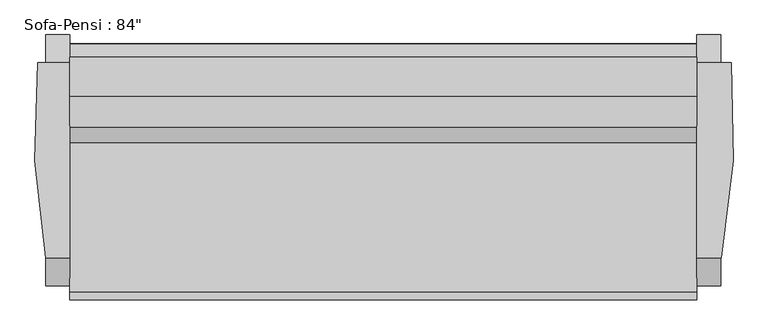
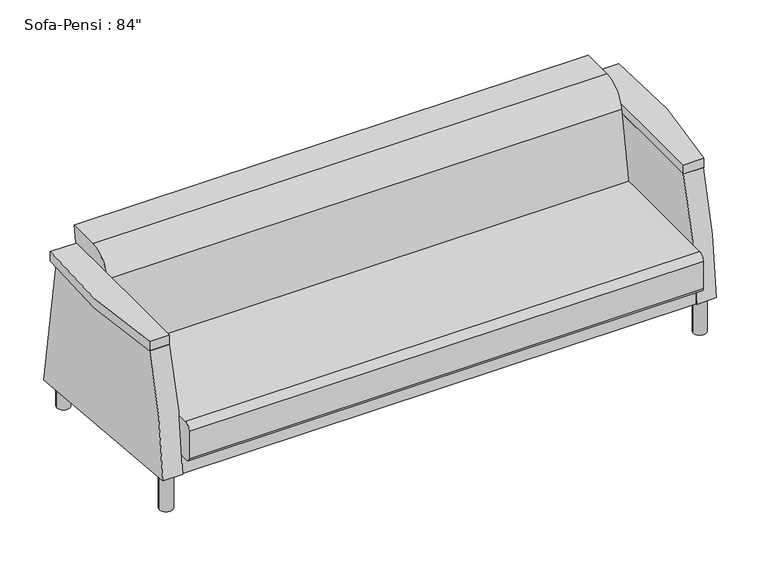
"""IFC4 building model written with IfcOpenShell, lengths in millimetres: furniture geometry."""

from ifc_helpers import new_model, si_unit, point, frame, frame_2d, origin, origin_with_axes, place, context, project, spatial, polyline, circle_curve, trimmed, segment, composite_curve, outline, extrude, source, transform, mapped, element, save


def furniture_4a9d42a7(model_context):
    return source(origin(), model_context, "Body", "SweptSolid", [
        extrude(outline(composite_curve([segment(trimmed(circle_curve(frame_2d((-116.5901639, 351.2509954)), 25.4), [point((-141.9901639, 351.2509954))], [point((-116.5901639, 376.6509954))], False, "CARTESIAN"), True, "CONTINUOUS"), segment(polyline([(-116.5901639, 376.6509954), (355.3895541, 376.6509954), (402.1988177, 642.1195211)]), True, "CONTINUOUS"), segment(trimmed(circle_curve(frame_2d((502.2552854, 624.4768662)), 101.6), [point((402.1988177, 642.1195211))], [point((502.2552854, 726.0768662))], False, "CARTESIAN"), True, "CONTINUOUS"), segment(polyline([(502.2552854, 726.0768662), (626.3344485, 726.0768662), (609.5377828, 620.1719187), (667.6541767, 224.2509954), (-126.1151639, 224.2509954)]), True, "CONTINUOUS"), segment(trimmed(circle_curve(frame_2d((-126.1151639, 240.1259954)), 15.875), [point((-126.1151639, 224.2509954))], [point((-141.9901639, 240.1259954))], False, "CARTESIAN"), True, "CONTINUOUS"), segment(polyline([(-141.9901639, 240.1259954), (-141.9901639, 351.2509954)]), True, "CONTINUOUS")], self_intersect=False)), frame((-711.99375, 0.0, 0.0), z_axis=(1.0, 0.0, 0.0), x_axis=(0.0, 1.0, 0.0)), (0.0, 0.0, 1.0), 1981.2),
        extrude(outline(composite_curve([segment(polyline([(696.2098361, 79.844579), (-97.7900405, 149.3105671)]), True, "CONTINUOUS"), segment(trimmed(circle_curve(frame_2d((1499.9783711, 99.5888442)), 1598.5418814), [point((-97.7900405, 149.3105671))], [point((-9.3943348, 626.0203985))], False, "CARTESIAN"), True, "CONTINUOUS"), segment(polyline([(-9.3943348, 626.0203985), (608.6917937, 626.0203985), (696.2098361, 79.844579)]), True, "CONTINUOUS")], self_intersect=False)), frame((1269.20625, 0.0, 0.0), z_axis=(1.0, 0.0, 0.0), x_axis=(0.0, 1.0, 0.0)), (0.0, 0.0, 1.0), 76.2),
        extrude(outline(composite_curve([segment(polyline([(-9.3943348, 626.0203985), (608.6917937, 626.0203985), (696.2098361, 79.844579), (-97.7900405, 149.3105671)]), True, "CONTINUOUS"), segment(trimmed(circle_curve(frame_2d((1499.9783711, 99.5888442)), 1598.5418814), [point((-97.7900405, 149.3105671))], [point((-9.3943348, 626.0203985))], False, "CARTESIAN"), True, "CONTINUOUS")], self_intersect=False)), frame((-788.19375, 0.0, 0.0), z_axis=(1.0, 0.0, 0.0), x_axis=(0.0, 1.0, 0.0)), (0.0, 0.0, 1.0), 76.2),
        extrude(outline(polyline([(1269.20625, 668.3047863), (1269.20625, -93.6952137), (-711.99375, -93.6952137), (-711.99375, 668.3047863), (1269.20625, 668.3047863)])), frame((0.0, 0.0, 148.0509954), z_axis=(0.0, 0.0, 1.0), x_axis=(1.0, 0.0, 0.0)), (0.0, 0.0, 1.0), 76.2),
        extrude(outline(composite_curve([segment(trimmed(circle_curve(frame_2d((-750.09375, -53.0901639)), 25.4), [point((-775.49375, -53.0901639))], [point((-724.69375, -53.0901639))], False, "CARTESIAN"), True, "CONTINUOUS"), segment(trimmed(circle_curve(frame_2d((-750.09375, -53.0901639)), 25.4), [point((-724.69375, -53.0901639))], [point((-775.49375, -53.0901639))], False, "CARTESIAN"), True, "CONTINUOUS")], self_intersect=False)), origin_with_axes(), (0.0, 0.0, 1.0), 148.43125),
        extrude(outline(composite_curve([segment(trimmed(circle_curve(frame_2d((-750.09375, 632.7098361)), 25.4), [point((-775.49375, 632.7098361))], [point((-724.69375, 632.7098361))], False, "CARTESIAN"), True, "CONTINUOUS"), segment(trimmed(circle_curve(frame_2d((-750.09375, 632.7098361)), 25.4), [point((-724.69375, 632.7098361))], [point((-775.49375, 632.7098361))], False, "CARTESIAN"), True, "CONTINUOUS")], self_intersect=False)), origin_with_axes(), (0.0, 0.0, 1.0), 148.43125),
        extrude(outline(composite_curve([segment(trimmed(circle_curve(frame_2d((1307.30625, 632.7098361)), 25.4), [point((1281.90625, 632.7098361))], [point((1332.70625, 632.7098361))], False, "CARTESIAN"), True, "CONTINUOUS"), segment(trimmed(circle_curve(frame_2d((1307.30625, 632.7098361)), 25.4), [point((1332.70625, 632.7098361))], [point((1281.90625, 632.7098361))], False, "CARTESIAN"), True, "CONTINUOUS")], self_intersect=False)), origin_with_axes(), (0.0, 0.0, 1.0), 148.43125),
        extrude(outline(composite_curve([segment(trimmed(circle_curve(frame_2d((1307.30625, -53.0901639)), 25.4), [point((1281.90625, -53.0901639))], [point((1332.70625, -53.0901639))], False, "CARTESIAN"), True, "CONTINUOUS"), segment(trimmed(circle_curve(frame_2d((1307.30625, -53.0901639)), 25.4), [point((1332.70625, -53.0901639))], [point((1281.90625, -53.0901639))], False, "CARTESIAN"), True, "CONTINUOUS")], self_intersect=False)), origin_with_axes(), (0.0, 0.0, 1.0), 148.43125),
        extrude(outline(composite_curve([segment(polyline([(-711.99375, -9.3943348), (-788.19375, -9.3943348)]), True, "CONTINUOUS"), segment(trimmed(circle_curve(frame_2d((1379.5527561, 389.2532985)), 2204.0972869), [point((-788.19375, -9.3943348))], [point((-813.59375, 608.6917935))], False, "CARTESIAN"), True, "CONTINUOUS"), segment(polyline([(-813.59375, 608.6917935), (-711.99375, 608.6917935), (-711.99375, -9.3943348)]), True, "CONTINUOUS")], self_intersect=False)), frame((0.0, 0.0, 626.0203985), z_axis=(0.0, 0.0, 1.0), x_axis=(1.0, 0.0, 0.0)), (0.0, 0.0, 1.0), 38.1),
        extrude(outline(composite_curve([segment(polyline([(1269.20625, -9.3943348), (1269.20625, 608.9395268), (1377.8864453, 608.9395268)]), True, "CONTINUOUS"), segment(trimmed(circle_curve(frame_2d((-821.3771494, 407.0073811)), 2208.514648), [point((1377.8864453, 608.9395268))], [point((1347.5273117, -9.3943348))], False, "CARTESIAN"), True, "CONTINUOUS"), segment(polyline([(1347.5273117, -9.3943348), (1269.20625, -9.3943348)]), True, "CONTINUOUS")], self_intersect=False)), frame((0.0, 0.0, 626.0203985), z_axis=(0.0, 0.0, 1.0), x_axis=(1.0, 0.0, 0.0)), (0.0, 0.0, 1.0), 38.1),
    ])


if __name__ == "__main__":
    model = new_model("IFC4")
    model_context = context("Model", 3, world=origin())
    ifc_project = project(units=[si_unit("LENGTHUNIT", "METRE", prefix="MILLI")], contexts=[model_context])
    site = spatial("IfcSite", under=ifc_project)
    building = spatial("IfcBuilding", under=site)
    placement = place(None, origin())
    furniture_shape = furniture_4a9d42a7(model_context)
    element("IfcFurniture", 1, ObjectType="Sofa-Pensi : 84\"", at=placement, inside=building, context=model_context, shape_type="MappedRepresentation", body=[
        mapped(furniture_shape, transform((0.0, 0.0, 0.0), x_axis=(1.0, 0.0, 0.0), y_axis=(0.0, 1.0, 0.0), z_axis=(0.0, 0.0, 1.0))),
    ])
    save(model, "model.ifc")

# Revit data of these elements
# Type "Sofa-Pensi : 84\""
#   Assembly Code = "E2020200"
#   Length = 7' - 0"
#   Frame Material = Cherry
#   Seat Material = Linen, Beige
#   Feet Material = Steel, Chrome Plated
#   Default Elevation = 0
# Element 1 (IfcFurniture, "Sofa-Pensi : 84\"")
#   Materials on its faces: "Cherry", "Linen, Beige", "Steel, Chrome Plated"
# Materials
#   "Cherry": class "Wood", colour RGB 226 177 128, transparency 0, Description = "Prunus Serotina", Cost = 0
#   "Linen, Beige": class "Textile", colour RGB 249 239 230, transparency 0, Description = "Linen, beige", Cost = 0
#   "Steel, Chrome Plated": class "Metal", colour RGB 17 17 17, transparency 0, Description = "Chromiuim plated steel", Cost = 0
